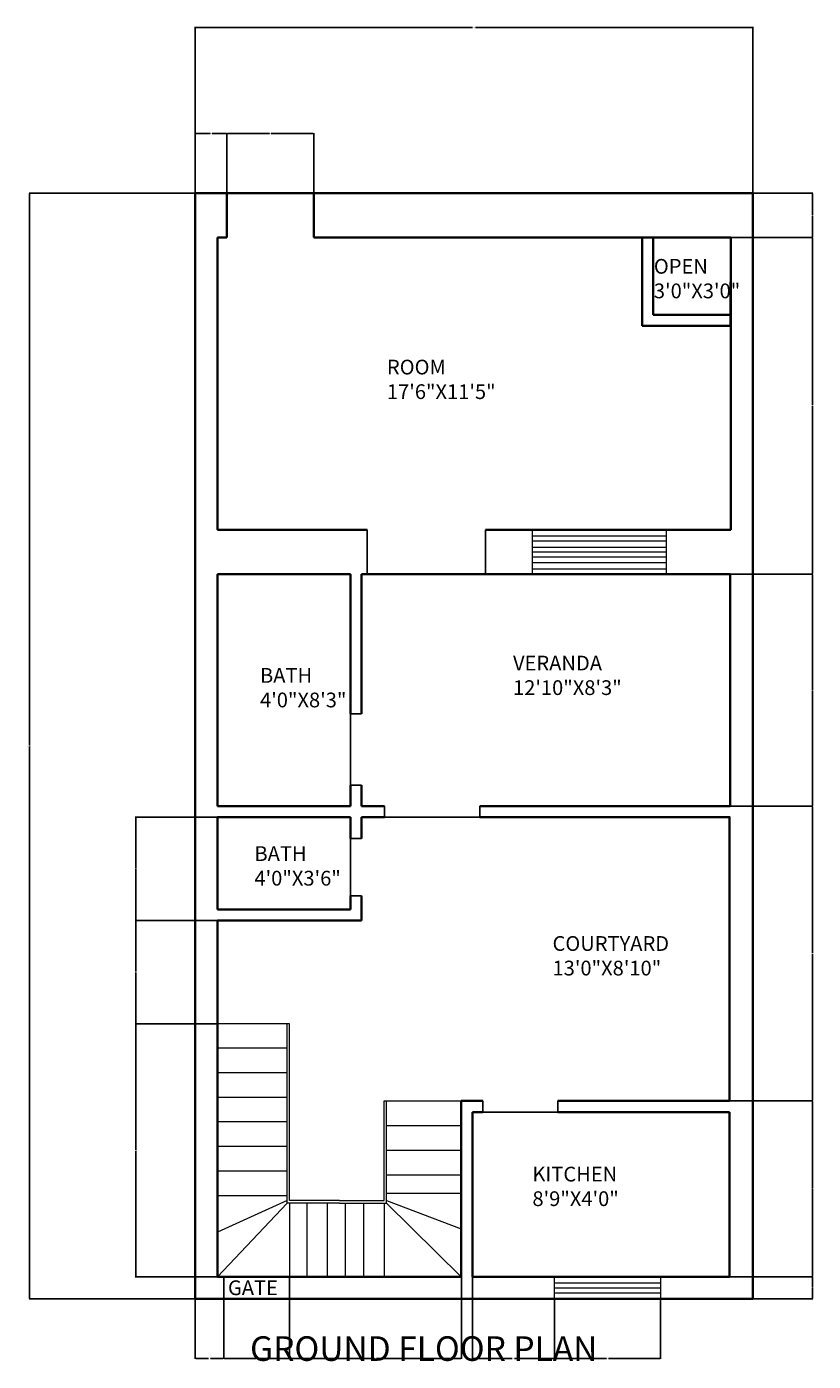
# Model space of a CAD drawing. Units: inches. Extents: x 2673 to 3344, y 1818 to 2362.
# Tile 1 of 2: x 2673 to 2994, y 1818 to 2362. Entities that reach past the tile are written whole.
import ezdxf

# ---------------------------------------------------------------- set-up
doc = ezdxf.new("R2010")
doc.units = ezdxf.units.IN
for name, color, linetype, lineweight in [('A-ANNO-DIMS', 2, 'Continuous', 18), ('A-ANNO-TEXT', 7, 'Continuous', 18), ('A-ANNO-TITL', 7, 'Continuous', 35), ('A-AREA-IDEN', 7, 'Continuous', 18), ('A-DOOR', 3, 'Continuous', 25), ('A-FLOR-STRS', 8, 'Continuous', 18), ('A-GLAZ', 4, 'Continuous', 18), ('A-WALL', 7, 'Continuous', 35)]:
    doc.layers.add(name, color=color, linetype=linetype, lineweight=lineweight)
doc.styles.get("Standard").update_dxf_attribs({"font": 'arial.ttf'})
doc.dimstyles.get("Standard").update_dxf_attribs({"dimtxt": 0.18, "dimasz": 0.18, "dimexe": 0.18, "dimexo": 0.0625, "dimgap": 0.09, "dimtad": 0, "dimtih": 1, "dimtoh": 1, "dimdec": 4, "dimzin": 0, "dimdsep": 46, "dimtxsty": 'Standard', "dimcen": 0.09, "dimadec": 0, "dimazin": 0, "dimtfac": 1, "dimtdec": 4, "dimtofl": 0, "dimtmove": 0, "dimatfit": 3, "dimfxl": 1, "dimtolj": 1, "dimtzin": 0, "dimarcsym": 0})

# ---------------------------------------------------------------- blocks, each defined once
blk = doc.blocks.new('FLOOR-PERIMETER-227X450')
for p, q in [((0, 450), (227, 450)), ((0, 0), (0, 450)), ((227, 450), (227, 0)), ((227, 0), (0, 0))]:
    blk.add_line(p, q)
blk = doc.blocks.new('*D2')
at = {"layer": 'A-ANNO-DIMS', "color": 0, "lineweight": -2, "transparency": 16777216}
for p, q in [((2742.07, 2293.79), (2674.46, 2293.79)), ((2674.64, 2293.61), (2674.64, 2068.98)), ((2674.64, 1843.97), (2674.64, 2068.61)), ((2742.07, 1843.79), (2674.46, 1843.79))]:
    blk.add_line(p, q, dxfattribs=at)
at = {"layer": 'A-ANNO-DIMS', "color": 0, "transparency": 16777216}
for points in [[(2674.61, 2293.61), (2674.67, 2293.61), (2674.64, 2293.79)], [(2674.61, 1843.97), (2674.67, 1843.97), (2674.64, 1843.79)]]:
    blk.add_solid(points, dxfattribs=at)
at = {"layer": 'Defpoints', "color": 0, "transparency": 16777216}
for p in [(2674.64, 2293.79), (2742.14, 2293.79), (2742.14, 1843.79)]:
    blk.add_point(p, dxfattribs=at)
at = {"layer": 'A-ANNO-DIMS', "color": 0, "transparency": 16777216, "insert": (2674.64, 2068.79), "char_height": 0.18, "attachment_point": 5}
blk.add_mtext('\\A1;FOOTPRINT 450 TYP.', dxfattribs=at)
blk = doc.blocks.new('*D3')
at = {"layer": 'A-ANNO-DIMS', "color": 0, "lineweight": -2, "transparency": 16777216}
for p, q in [((2742.14, 2293.86), (2742.14, 2361.47)), ((2742.32, 2361.29), (2855.04, 2361.29)), ((2968.96, 2361.29), (2856.24, 2361.29)), ((2969.14, 2293.86), (2969.14, 2361.47))]:
    blk.add_line(p, q, dxfattribs=at)
at = {"layer": 'A-ANNO-DIMS', "color": 0, "transparency": 16777216}
for points in [[(2742.32, 2361.32), (2742.32, 2361.26), (2742.14, 2361.29)], [(2968.96, 2361.32), (2968.96, 2361.26), (2969.14, 2361.29)]]:
    blk.add_solid(points, dxfattribs=at)
at = {"layer": 'Defpoints', "color": 0, "transparency": 16777216}
for p in [(2969.14, 2361.29), (2742.14, 2293.79), (2969.14, 2293.79)]:
    blk.add_point(p, dxfattribs=at)
at = {"layer": 'A-ANNO-DIMS', "color": 0, "transparency": 16777216, "insert": (2855.64, 2361.29), "char_height": 0.18, "attachment_point": 5}
blk.add_mtext('\\A1;227 TYP.', dxfattribs=at)
blk = doc.blocks.new('*D6')
at = {"layer": 'A-ANNO-DIMS', "color": 0, "lineweight": -2, "transparency": 16777216}
for p, q in [((2959.72, 1852.79), (2993.57, 1852.79)), ((2993.39, 1852.61), (2993.39, 1848.48)), ((2993.39, 1843.97), (2993.39, 1848.11)), ((2969.2, 1843.79), (2993.57, 1843.79))]:
    blk.add_line(p, q, dxfattribs=at)
at = {"layer": 'A-ANNO-DIMS', "color": 0, "transparency": 16777216}
for points in [[(2993.36, 1852.61), (2993.42, 1852.61), (2993.39, 1852.79)], [(2993.36, 1843.97), (2993.42, 1843.97), (2993.39, 1843.79)]]:
    blk.add_solid(points, dxfattribs=at)
at = {"layer": 'Defpoints', "color": 0, "transparency": 16777216}
for p in [(2959.65, 1852.79), (2993.39, 1852.79), (2969.14, 1843.79)]:
    blk.add_point(p, dxfattribs=at)
at = {"layer": 'A-ANNO-DIMS', "color": 0, "transparency": 16777216, "insert": (2993.39, 1848.29), "char_height": 0.18, "attachment_point": 5}
blk.add_mtext('\\A1;9', dxfattribs=at)
blk = doc.blocks.new('*D7')
at = {"layer": 'A-ANNO-DIMS', "color": 0, "lineweight": -2, "transparency": 16777216}
for p, q in [((2959.72, 1924.35), (2993.57, 1924.35)), ((2993.39, 1924.17), (2993.39, 1888.75)), ((2993.39, 1852.97), (2993.39, 1888.39)), ((2959.72, 1852.79), (2993.57, 1852.79))]:
    blk.add_line(p, q, dxfattribs=at)
at = {"layer": 'A-ANNO-DIMS', "color": 0, "transparency": 16777216}
for points in [[(2993.36, 1924.17), (2993.42, 1924.17), (2993.39, 1924.35)], [(2993.36, 1852.97), (2993.42, 1852.97), (2993.39, 1852.79)]]:
    blk.add_solid(points, dxfattribs=at)
at = {"layer": 'Defpoints', "color": 0, "transparency": 16777216}
for p in [(2959.65, 1924.35), (2993.39, 1924.35), (2959.65, 1852.79)]:
    blk.add_point(p, dxfattribs=at)
at = {"layer": 'A-ANNO-DIMS', "color": 0, "transparency": 16777216, "insert": (2993.39, 1888.57), "char_height": 0.18, "attachment_point": 5}
blk.add_mtext('\\A1;71.55', dxfattribs=at)
blk = doc.blocks.new('*D8')
at = {"layer": 'A-ANNO-DIMS', "color": 0, "lineweight": -2, "transparency": 16777216}
for p, q in [((2960.01, 2044.3), (2993.57, 2044.3)), ((2993.39, 2044.12), (2993.39, 1984.5)), ((2993.39, 1924.53), (2993.39, 1984.14)), ((2959.72, 1924.35), (2993.57, 1924.35))]:
    blk.add_line(p, q, dxfattribs=at)
at = {"layer": 'A-ANNO-DIMS', "color": 0, "transparency": 16777216}
for points in [[(2993.36, 2044.12), (2993.42, 2044.12), (2993.39, 2044.3)], [(2993.36, 1924.53), (2993.42, 1924.53), (2993.39, 1924.35)]]:
    blk.add_solid(points, dxfattribs=at)
at = {"layer": 'Defpoints', "color": 0, "transparency": 16777216}
for p in [(2959.95, 2044.3), (2993.39, 2044.3), (2959.65, 1924.35)]:
    blk.add_point(p, dxfattribs=at)
at = {"layer": 'A-ANNO-DIMS', "color": 0, "transparency": 16777216, "insert": (2993.39, 1984.32), "char_height": 0.18, "attachment_point": 5}
blk.add_mtext('\\A1;119.95', dxfattribs=at)
blk = doc.blocks.new('*D9')
at = {"layer": 'A-ANNO-DIMS', "color": 0, "lineweight": -2, "transparency": 16777216}
for p, q in [((2960.01, 2138.79), (2993.57, 2138.79)), ((2993.39, 2138.61), (2993.39, 2091.73)), ((2993.39, 2044.48), (2993.39, 2091.36)), ((2960.01, 2044.3), (2993.57, 2044.3))]:
    blk.add_line(p, q, dxfattribs=at)
at = {"layer": 'A-ANNO-DIMS', "color": 0, "transparency": 16777216}
for points in [[(2993.36, 2138.61), (2993.42, 2138.61), (2993.39, 2138.79)], [(2993.36, 2044.48), (2993.42, 2044.48), (2993.39, 2044.3)]]:
    blk.add_solid(points, dxfattribs=at)
at = {"layer": 'Defpoints', "color": 0, "transparency": 16777216}
for p in [(2959.95, 2138.79), (2993.39, 2138.79), (2959.95, 2044.3)]:
    blk.add_point(p, dxfattribs=at)
at = {"layer": 'A-ANNO-DIMS', "color": 0, "transparency": 16777216, "insert": (2993.39, 2091.55), "char_height": 0.18, "attachment_point": 5}
blk.add_mtext('\\A1;94.5', dxfattribs=at)
blk = doc.blocks.new('*D10')
at = {"layer": 'A-ANNO-DIMS', "color": 0, "lineweight": -2, "transparency": 16777216}
for p, q in [((2960.2, 2275.79), (2993.57, 2275.79)), ((2993.39, 2275.61), (2993.39, 2207.48)), ((2993.39, 2138.97), (2993.39, 2207.11)), ((2960.01, 2138.79), (2993.57, 2138.79))]:
    blk.add_line(p, q, dxfattribs=at)
at = {"layer": 'A-ANNO-DIMS', "color": 0, "transparency": 16777216}
for points in [[(2993.36, 2275.61), (2993.42, 2275.61), (2993.39, 2275.79)], [(2993.36, 2138.97), (2993.42, 2138.97), (2993.39, 2138.79)]]:
    blk.add_solid(points, dxfattribs=at)
at = {"layer": 'Defpoints', "color": 0, "transparency": 16777216}
for p in [(2960.14, 2275.79), (2993.39, 2275.79), (2959.95, 2138.79)]:
    blk.add_point(p, dxfattribs=at)
at = {"layer": 'A-ANNO-DIMS', "color": 0, "transparency": 16777216, "insert": (2993.39, 2207.29), "char_height": 0.18, "attachment_point": 5}
blk.add_mtext('\\A1;137', dxfattribs=at)
blk = doc.blocks.new('*D11')
at = {"layer": 'A-ANNO-DIMS', "color": 0, "lineweight": -2, "transparency": 16777216}
for p, q in [((2969.2, 2293.79), (2993.57, 2293.79)), ((2993.39, 2293.61), (2993.39, 2284.98)), ((2993.39, 2275.97), (2993.39, 2284.61)), ((2960.2, 2275.79), (2993.57, 2275.79))]:
    blk.add_line(p, q, dxfattribs=at)
at = {"layer": 'A-ANNO-DIMS', "color": 0, "transparency": 16777216}
for points in [[(2993.36, 2293.61), (2993.42, 2293.61), (2993.39, 2293.79)], [(2993.36, 2275.97), (2993.42, 2275.97), (2993.39, 2275.79)]]:
    blk.add_solid(points, dxfattribs=at)
at = {"layer": 'Defpoints', "color": 0, "transparency": 16777216}
for p in [(2969.14, 2293.79), (2993.39, 2293.79), (2960.14, 2275.79)]:
    blk.add_point(p, dxfattribs=at)
at = {"layer": 'A-ANNO-DIMS', "color": 0, "transparency": 16777216, "insert": (2993.39, 2284.79), "char_height": 0.18, "attachment_point": 5}
blk.add_mtext('\\A1;18', dxfattribs=at)
blk = doc.blocks.new('*D12')
at = {"layer": 'A-ANNO-DIMS', "color": 0, "lineweight": -2, "transparency": 16777216}
for p, q in [((2742.14, 1843.73), (2742.14, 1819.36)), ((2753.69, 1843.73), (2753.69, 1819.36)), ((2742.32, 1819.54), (2747.46, 1819.54)), ((2753.51, 1819.54), (2748.37, 1819.54))]:
    blk.add_line(p, q, dxfattribs=at)
at = {"layer": 'A-ANNO-DIMS', "color": 0, "transparency": 16777216}
for points in [[(2742.32, 1819.57), (2742.32, 1819.51), (2742.14, 1819.54)], [(2753.51, 1819.57), (2753.51, 1819.51), (2753.69, 1819.54)]]:
    blk.add_solid(points, dxfattribs=at)
at = {"layer": 'Defpoints', "color": 0, "transparency": 16777216}
for p in [(2742.14, 1843.79), (2753.69, 1843.79), (2753.69, 1819.54)]:
    blk.add_point(p, dxfattribs=at)
at = {"layer": 'A-ANNO-DIMS', "color": 0, "transparency": 16777216, "insert": (2747.91, 1819.54), "char_height": 0.18, "attachment_point": 5}
blk.add_mtext('\\A1;11.556', dxfattribs=at)
blk = doc.blocks.new('*D13')
at = {"layer": 'A-ANNO-DIMS', "color": 0, "lineweight": -2, "transparency": 16777216}
for p, q in [((2753.69, 1843.73), (2753.69, 1819.36)), ((2780.49, 1843.73), (2780.49, 1819.36)), ((2753.87, 1819.54), (2766.77, 1819.54)), ((2780.31, 1819.54), (2767.42, 1819.54))]:
    blk.add_line(p, q, dxfattribs=at)
at = {"layer": 'A-ANNO-DIMS', "color": 0, "transparency": 16777216}
for points in [[(2753.87, 1819.57), (2753.87, 1819.51), (2753.69, 1819.54)], [(2780.31, 1819.57), (2780.31, 1819.51), (2780.49, 1819.54)]]:
    blk.add_solid(points, dxfattribs=at)
at = {"layer": 'Defpoints', "color": 0, "transparency": 16777216}
for p in [(2753.69, 1843.79), (2780.49, 1843.79), (2780.49, 1819.54)]:
    blk.add_point(p, dxfattribs=at)
at = {"layer": 'A-ANNO-DIMS', "color": 0, "transparency": 16777216, "insert": (2767.09, 1819.54), "char_height": 0.18, "attachment_point": 5}
blk.add_mtext('\\A1;26.8', dxfattribs=at)
blk = doc.blocks.new('*D14')
at = {"layer": 'A-ANNO-DIMS', "color": 0, "lineweight": -2, "transparency": 16777216}
for p, q in [((2850.45, 1852.73), (2850.45, 1819.36)), ((2780.49, 1843.73), (2780.49, 1819.36)), ((2780.67, 1819.54), (2815.08, 1819.54)), ((2850.27, 1819.54), (2815.86, 1819.54))]:
    blk.add_line(p, q, dxfattribs=at)
at = {"layer": 'A-ANNO-DIMS', "color": 0, "transparency": 16777216}
for points in [[(2780.67, 1819.57), (2780.67, 1819.51), (2780.49, 1819.54)], [(2850.27, 1819.57), (2850.27, 1819.51), (2850.45, 1819.54)]]:
    blk.add_solid(points, dxfattribs=at)
at = {"layer": 'Defpoints', "color": 0, "transparency": 16777216}
for p in [(2850.45, 1852.79), (2780.49, 1843.79), (2850.45, 1819.54)]:
    blk.add_point(p, dxfattribs=at)
at = {"layer": 'A-ANNO-DIMS', "color": 0, "transparency": 16777216, "insert": (2815.47, 1819.54), "char_height": 0.18, "attachment_point": 5}
blk.add_mtext('\\A1;69.95', dxfattribs=at)
blk = doc.blocks.new('*D15')
at = {"layer": 'A-ANNO-DIMS', "color": 0, "lineweight": -2, "transparency": 16777216}
for p, q in [((2854.95, 1852.73), (2854.95, 1819.36)), ((2888.33, 1843.73), (2888.33, 1819.36)), ((2855.13, 1819.54), (2871.18, 1819.54)), ((2888.15, 1819.54), (2872.1, 1819.54))]:
    blk.add_line(p, q, dxfattribs=at)
at = {"layer": 'A-ANNO-DIMS', "color": 0, "transparency": 16777216}
for points in [[(2855.13, 1819.57), (2855.13, 1819.51), (2854.95, 1819.54)], [(2888.15, 1819.57), (2888.15, 1819.51), (2888.33, 1819.54)]]:
    blk.add_solid(points, dxfattribs=at)
at = {"layer": 'Defpoints', "color": 0, "transparency": 16777216}
for p in [(2854.95, 1852.79), (2888.33, 1843.79), (2888.33, 1819.54)]:
    blk.add_point(p, dxfattribs=at)
at = {"layer": 'A-ANNO-DIMS', "color": 0, "transparency": 16777216, "insert": (2871.64, 1819.54), "char_height": 0.18, "attachment_point": 5}
blk.add_mtext('\\A1;33.386', dxfattribs=at)
blk = doc.blocks.new('*D16')
at = {"layer": 'A-ANNO-DIMS', "color": 0, "lineweight": -2, "transparency": 16777216}
for p, q in [((2888.33, 1843.73), (2888.33, 1819.36)), ((2931.58, 1843.73), (2931.58, 1819.36)), ((2888.51, 1819.54), (2909.49, 1819.54)), ((2931.4, 1819.54), (2910.42, 1819.54))]:
    blk.add_line(p, q, dxfattribs=at)
at = {"layer": 'A-ANNO-DIMS', "color": 0, "transparency": 16777216}
for points in [[(2888.51, 1819.57), (2888.51, 1819.51), (2888.33, 1819.54)], [(2931.4, 1819.57), (2931.4, 1819.51), (2931.58, 1819.54)]]:
    blk.add_solid(points, dxfattribs=at)
at = {"layer": 'Defpoints', "color": 0, "transparency": 16777216}
for p in [(2888.33, 1843.79), (2931.58, 1843.79), (2931.58, 1819.54)]:
    blk.add_point(p, dxfattribs=at)
at = {"layer": 'A-ANNO-DIMS', "color": 0, "transparency": 16777216, "insert": (2909.96, 1819.54), "char_height": 0.18, "attachment_point": 5}
blk.add_mtext('\\A1;43.245', dxfattribs=at)
blk = doc.blocks.new('*D17')
at = {"layer": 'A-ANNO-DIMS', "color": 0, "lineweight": -2, "transparency": 16777216}
for p, q in [((2742.14, 2293.86), (2742.14, 2318.22)), ((2742.32, 2318.04), (2748.12, 2318.04)), ((2754.84, 2318.04), (2749.03, 2318.04)), ((2755.02, 2293.86), (2755.02, 2318.22))]:
    blk.add_line(p, q, dxfattribs=at)
at = {"layer": 'A-ANNO-DIMS', "color": 0, "transparency": 16777216}
for points in [[(2742.32, 2318.07), (2742.32, 2318.01), (2742.14, 2318.04)], [(2754.84, 2318.07), (2754.84, 2318.01), (2755.02, 2318.04)]]:
    blk.add_solid(points, dxfattribs=at)
at = {"layer": 'Defpoints', "color": 0, "transparency": 16777216}
for p in [(2755.02, 2318.04), (2742.14, 2293.79), (2755.02, 2293.79)]:
    blk.add_point(p, dxfattribs=at)
at = {"layer": 'A-ANNO-DIMS', "color": 0, "transparency": 16777216, "insert": (2748.58, 2318.04), "char_height": 0.18, "attachment_point": 5}
blk.add_mtext('\\A1;12.884', dxfattribs=at)
blk = doc.blocks.new('*D18')
at = {"layer": 'A-ANNO-DIMS', "color": 0, "lineweight": -2, "transparency": 16777216}
for p, q in [((2755.02, 2293.86), (2755.02, 2318.22)), ((2755.2, 2318.04), (2772.3, 2318.04)), ((2790.15, 2318.04), (2773.05, 2318.04)), ((2790.33, 2293.86), (2790.33, 2318.22))]:
    blk.add_line(p, q, dxfattribs=at)
at = {"layer": 'A-ANNO-DIMS', "color": 0, "transparency": 16777216}
for points in [[(2755.2, 2318.07), (2755.2, 2318.01), (2755.02, 2318.04)], [(2790.15, 2318.07), (2790.15, 2318.01), (2790.33, 2318.04)]]:
    blk.add_solid(points, dxfattribs=at)
at = {"layer": 'Defpoints', "color": 0, "transparency": 16777216}
for p in [(2790.33, 2318.04), (2755.02, 2293.79), (2790.33, 2293.79)]:
    blk.add_point(p, dxfattribs=at)
at = {"layer": 'A-ANNO-DIMS', "color": 0, "transparency": 16777216, "insert": (2772.68, 2318.04), "char_height": 0.18, "attachment_point": 5}
blk.add_mtext('\\A1;35.31', dxfattribs=at)
blk = doc.blocks.new('*D19')
at = {"layer": 'A-ANNO-DIMS', "color": 0, "lineweight": -2, "transparency": 16777216}
for p, q in [((2751.07, 1955.8), (2717.71, 1955.8)), ((2717.89, 1955.62), (2717.89, 1904.48)), ((2717.89, 1852.97), (2717.89, 1904.11)), ((2751.07, 1852.79), (2717.71, 1852.79))]:
    blk.add_line(p, q, dxfattribs=at)
at = {"layer": 'A-ANNO-DIMS', "color": 0, "transparency": 16777216}
for points in [[(2717.86, 1955.62), (2717.92, 1955.62), (2717.89, 1955.8)], [(2717.86, 1852.97), (2717.92, 1852.97), (2717.89, 1852.79)]]:
    blk.add_solid(points, dxfattribs=at)
at = {"layer": 'Defpoints', "color": 0, "transparency": 16777216}
for p in [(2717.89, 1955.8), (2751.14, 1955.8), (2751.14, 1852.79)]:
    blk.add_point(p, dxfattribs=at)
at = {"layer": 'A-ANNO-DIMS', "color": 0, "transparency": 16777216, "insert": (2717.89, 1904.3), "char_height": 0.18, "attachment_point": 5}
blk.add_mtext('\\A1;103', dxfattribs=at)
blk = doc.blocks.new('*D20')
at = {"layer": 'A-ANNO-DIMS', "color": 0, "lineweight": -2, "transparency": 16777216}
for p, q in [((2751.07, 1997.8), (2717.71, 1997.8)), ((2717.89, 1997.62), (2717.89, 1976.98)), ((2717.89, 1955.98), (2717.89, 1976.62)), ((2751.07, 1955.8), (2717.71, 1955.8))]:
    blk.add_line(p, q, dxfattribs=at)
at = {"layer": 'A-ANNO-DIMS', "color": 0, "transparency": 16777216}
for points in [[(2717.86, 1997.62), (2717.92, 1997.62), (2717.89, 1997.8)], [(2717.86, 1955.98), (2717.92, 1955.98), (2717.89, 1955.8)]]:
    blk.add_solid(points, dxfattribs=at)
at = {"layer": 'Defpoints', "color": 0, "transparency": 16777216}
for p in [(2717.89, 1997.8), (2751.14, 1997.8), (2751.14, 1955.8)]:
    blk.add_point(p, dxfattribs=at)
at = {"layer": 'A-ANNO-DIMS', "color": 0, "transparency": 16777216, "insert": (2717.89, 1976.8), "char_height": 0.18, "attachment_point": 5}
blk.add_mtext('\\A1;42', dxfattribs=at)
blk = doc.blocks.new('*D21')
at = {"layer": 'A-ANNO-DIMS', "color": 0, "lineweight": -2, "transparency": 16777216}
for p, q in [((2751.07, 2039.8), (2717.71, 2039.8)), ((2717.89, 2039.62), (2717.89, 2018.98)), ((2717.89, 1997.98), (2717.89, 2018.62)), ((2751.07, 1997.8), (2717.71, 1997.8))]:
    blk.add_line(p, q, dxfattribs=at)
at = {"layer": 'A-ANNO-DIMS', "color": 0, "transparency": 16777216}
for points in [[(2717.86, 2039.62), (2717.92, 2039.62), (2717.89, 2039.8)], [(2717.86, 1997.98), (2717.92, 1997.98), (2717.89, 1997.8)]]:
    blk.add_solid(points, dxfattribs=at)
at = {"layer": 'Defpoints', "color": 0, "transparency": 16777216}
for p in [(2717.89, 2039.8), (2751.14, 2039.8), (2751.14, 1997.8)]:
    blk.add_point(p, dxfattribs=at)
at = {"layer": 'A-ANNO-DIMS', "color": 0, "transparency": 16777216, "insert": (2717.89, 2018.8), "char_height": 0.18, "attachment_point": 5}
blk.add_mtext('\\A1;42', dxfattribs=at)

msp = doc.modelspace()

# ---------------------------------------------------------------- linework, layer by layer
at = {"layer": 'A-DOOR'}
for p, q in [((2812.0877, 2138.7941), (2812.0877, 2156.7941)), ((2860.2455, 2138.7941), (2860.2455, 2156.7941)), ((2805.3617, 2081.8721), (2809.8617, 2081.8721)), ((2805.3617, 2081.8721), (2805.3617, 2052.8408)), ((2805.3617, 2052.8408), (2809.8617, 2052.8408)), ((2819.1101, 2039.7972), (2819.1101, 2044.2972)), ((2857.9709, 2039.7972), (2857.9709, 2044.2972)), ((2819.1101, 2039.7972), (2857.9709, 2039.7972)), ((2805.3617, 2031.1818), (2809.8617, 2031.1818)), ((2805.3617, 2007.8792), (2805.3617, 2031.1818)), ((2805.3617, 2007.8792), (2809.8617, 2007.8792)), ((2859.1524, 1919.8472), (2859.1524, 1924.3472)), ((2889.7363, 1919.8472), (2889.7363, 1924.3472)), ((2859.1524, 1919.8472), (2890.9676, 1919.8472)), ((2753.6928, 1852.7936), (2753.6928, 1843.7936)), ((2780.4931, 1852.7936), (2780.4931, 1843.7936))]:
    msp.add_line(p, q, dxfattribs=at)
at = {"layer": 'A-FLOR-STRS'}
for p, q in [((2780.4931, 1955.7975), (2751.137, 1955.7975)), ((2779.4931, 1924.3472), (2779.4931, 1955.7975)), ((2780.4931, 1924.3472), (2780.4931, 1955.7975)), ((2779.4931, 1945.7975), (2751.137, 1945.7975)), ((2779.4931, 1935.7975), (2751.137, 1935.7975)), ((2779.4931, 1925.7975), (2751.137, 1925.7975)), ((2779.4931, 1882.7728), (2779.4931, 1924.3472)), ((2780.4931, 1883.7728), (2780.4931, 1924.3472)), ((2818.9849, 1883.7728), (2818.9849, 1924.3472)), ((2818.9849, 1924.3472), (2819.9849, 1924.3472)), ((2819.9849, 1882.7728), (2819.9849, 1924.3472)), ((2819.9849, 1924.3472), (2850.4469, 1924.3472)), ((2779.4931, 1915.7975), (2751.137, 1915.7975)), ((2819.9849, 1914.3472), (2850.4469, 1914.3472)), ((2779.4931, 1905.7975), (2751.137, 1905.7975)), ((2819.9849, 1904.3472), (2850.4469, 1904.3472)), ((2779.4931, 1895.7975), (2751.137, 1895.7975)), ((2819.9849, 1894.3472), (2850.4469, 1894.3472)), ((2779.4931, 1885.7975), (2751.137, 1885.7975)), ((2819.9849, 1886.8433), (2850.4469, 1886.8433)), ((2779.4931, 1883.7728), (2751.137, 1870.992)), ((2779.4931, 1882.7728), (2751.137, 1852.7936)), ((2800.792, 1882.7728), (2779.4931, 1882.7728)), ((2800.792, 1883.7728), (2780.4931, 1883.7728)), ((2780.4931, 1882.7728), (2780.4931, 1852.7936)), ((2787.7372, 1852.7936), (2787.7372, 1882.7728)), ((2795.9322, 1852.7936), (2795.9322, 1882.7728)), ((2800.792, 1883.7728), (2818.9849, 1883.7728)), ((2800.792, 1882.7728), (2819.9849, 1882.7728)), ((2803.2385, 1852.7936), (2803.2385, 1882.7728)), ((2810.7424, 1852.7936), (2810.7424, 1882.7728)), ((2818.9849, 1882.7728), (2818.9849, 1852.7936)), ((2819.9849, 1883.7728), (2850.4469, 1872.2734)), ((2819.9849, 1882.7728), (2850.4469, 1852.7907))]:
    msp.add_line(p, q, dxfattribs=at)
at = {"layer": 'A-GLAZ'}
for p, q in [((2879.3937, 2154.389), (2933.8124, 2154.389)), ((2879.3937, 2152.3252), (2933.8124, 2152.3252)), ((2879.3937, 2149.7455), (2933.8124, 2149.7455)), ((2879.3937, 2147.7941), (2933.8124, 2147.7941)), ((2879.3937, 2145.8621), (2933.8124, 2145.8621)), ((2879.3937, 2143.5352), (2933.8124, 2143.5352)), ((2879.3937, 2140.8851), (2933.8124, 2140.8851)), ((2888.3325, 1850.2838), (2931.5776, 1850.3475)), ((2888.3325, 1848.2936), (2931.5776, 1848.2936)), ((2888.3325, 1846.2746), (2931.5776, 1846.2746))]:
    msp.add_line(p, q, dxfattribs=at)
for points in [[(2879.3937, 2156.7941), (2933.8124, 2156.7941), (2933.8124, 2138.7941), (2879.3937, 2138.7941)], [(2888.3325, 1852.7936), (2931.5776, 1852.7936), (2931.5776, 1843.7936), (2888.3325, 1843.7936)]]:
    msp.add_lwpolyline(points, close=True, dxfattribs=at)
at = {"layer": 'A-WALL'}
for p, q in [((2755.0211, 2275.7936), (2755.0211, 2293.7936)), ((2790.3344, 2275.7936), (2790.3344, 2293.7936)), ((2751.137, 2275.7936), (2755.0211, 2275.7936)), ((2751.137, 2156.7941), (2751.137, 2275.7936)), ((2790.3344, 2275.7936), (2960.137, 2275.7936)), ((2924.0554, 2239.7937), (2924.0554, 2275.7936)), ((2928.5554, 2244.2937), (2928.5554, 2275.7936)), ((2960.137, 2275.7936), (2960.0554, 2239.7937)), ((2960.137, 2275.7936), (2960.137, 2156.7941)), ((2960.0554, 2244.2937), (2928.5554, 2244.2937)), ((2960.0554, 2239.7937), (2924.0554, 2239.7937)), ((2809.4189, 2156.7941), (2751.137, 2156.7941)), ((2809.8617, 2156.7941), (2809.4189, 2156.7941)), ((2812.0877, 2156.7941), (2809.8617, 2156.7941)), ((2959.7568, 2156.7941), (2860.2455, 2156.7941)), ((2959.7568, 2156.7941), (2960.137, 2156.7941)), ((2805.3617, 2138.7941), (2751.137, 2138.7941)), ((2751.137, 2044.2972), (2751.137, 2138.7941)), ((2805.3617, 2081.8721), (2805.3617, 2138.7941)), ((2809.8617, 2138.7941), (2860.2455, 2138.7941)), ((2809.8617, 2081.8721), (2809.8617, 2138.7941)), ((2959.7568, 2138.7941), (2860.2455, 2138.7941)), ((2959.7568, 2138.7941), (2959.9469, 2138.7941)), ((2959.9469, 2138.7941), (2959.9469, 2044.2972)), ((2805.3617, 2044.2972), (2805.3617, 2052.8408)), ((2809.8617, 2044.2972), (2809.8617, 2052.8408)), ((2805.3617, 2044.2972), (2751.137, 2044.2972)), ((2819.1101, 2044.2972), (2809.8617, 2044.2972)), ((2959.3617, 2044.2972), (2857.9709, 2044.2972)), ((2959.3617, 2044.2972), (2959.9469, 2044.2972)), ((2805.3617, 2039.7972), (2751.137, 2039.7972)), ((2751.137, 2002.2983), (2751.137, 2039.7972)), ((2805.3617, 2039.7972), (2805.3617, 2031.1818)), ((2809.8617, 2039.7972), (2809.8617, 2031.1818)), ((2819.1101, 2039.7972), (2809.8617, 2039.7972)), ((2959.3617, 2039.7972), (2857.9709, 2039.7972)), ((2959.3617, 2039.7972), (2959.9469, 2039.7972)), ((2959.6543, 2039.7972), (2959.6543, 1924.3472)), ((2805.3617, 2007.8792), (2805.3617, 2002.2983)), ((2809.8617, 2007.8792), (2809.8617, 1997.7983)), ((2805.0541, 2002.2983), (2751.137, 2002.2983)), ((2805.0541, 2002.2983), (2805.3617, 2002.2983)), ((2751.137, 1852.7936), (2751.137, 1997.7983)), ((2805.0541, 1997.7983), (2751.137, 1997.7983)), ((2805.0541, 1997.7983), (2805.3617, 1997.7983)), ((2805.3617, 1997.7983), (2809.8617, 1997.7983)), ((2850.4469, 1919.8472), (2850.4469, 1924.3472)), ((2859.1524, 1924.3472), (2850.4469, 1924.3472)), ((2959.6543, 1924.3472), (2889.7363, 1924.3472)), ((2850.4469, 1852.7907), (2850.4469, 1919.8472)), ((2854.9469, 1852.7907), (2854.9469, 1919.8472)), ((2859.1524, 1919.8472), (2854.9469, 1919.8472)), ((2959.6543, 1919.8472), (2889.7363, 1919.8472)), ((2959.6543, 1919.8472), (2959.6543, 1852.7936)), ((2850.4469, 1852.7936), (2751.137, 1852.7936)), ((2959.6543, 1852.7936), (2854.9469, 1852.7936))]:
    msp.add_line(p, q, dxfattribs=at)

# ---------------------------------------------------------------- block references
msp.add_blockref('FLOOR-PERIMETER-227X450', (2742.137, 1843.7936), dxfattribs=at)

# ---------------------------------------------------------------- texts
at = {"layer": 'A-ANNO-TEXT', "insert": (2755.4278, 1851.3267), "char_height": 6, "attachment_point": 1}
msp.add_mtext_dynamic_manual_height_columns('GATE\\P ', width=4.95123, gutter_width=12.5, heights=[0], dxfattribs=at)
at = {"layer": 'A-ANNO-TITL', "insert": (2764.4221, 1828.5696), "char_height": 10, "attachment_point": 1}
msp.add_mtext_dynamic_manual_height_columns('GROUND FLOOR PLAN ', width=156.994222, gutter_width=12.5, heights=[0], dxfattribs=at)
at = {"layer": 'A-AREA-IDEN', "char_height": 6, "attachment_point": 1}
for s, width, insert in [('OPEN\\P3\'0"X3\'0"', 7.792091, (2928.8408, 2267.0357)), ('ROOM \\P17\'6"X11\'5"', 44.612926, (2820.1518, 2226.0263)), ('VERANDA\\P12\'10"X8\'3"', 37.705968, (2871.4973, 2105.5668)), ('BATH\\P4\'0"X8\'3"', 10.849641, (2768.4898, 2100.5464)), ('BATH\\P4\'0"X3\'6"', 10.849641, (2766.2121, 2028.0119)), ('COURTYARD\\P13\'0"X8\'10"', 22.904962, (2887.5788, 1991.4332)), ('KITCHEN \\P8\'9"X4\'0"', 28.845327, (2879.3946, 1897.579))]:
    msp.add_mtext_dynamic_manual_height_columns(s, width=width, gutter_width=12.5, heights=[0], dxfattribs=dict(at, insert=insert))

# ---------------------------------------------------------------- dimensions: what is measured, and where the dimension line sits
at = {"layer": 'A-ANNO-DIMS'}
dim = msp.add_linear_dim(base=(2969.137, 2361.2936), p1=(2742.137, 2293.7936), p2=(2969.137, 2293.7936), text='<> TYP.', dimstyle='Standard', override={"dimdec": 0, "dimlfac": 1, "dimrnd": 0, "dimzin": 0, "dimdsep": 46, "dimlunit": 2}, dxfattribs=at)
dim.commit()
dim.dimension.update_dxf_attribs({"geometry": '*D3', "text_midpoint": (2855.637, 2361.2936)})
for base, p1, p2, override, picture, middle in [((2755.0211, 2318.0436), (2742.137, 2293.7936), (2755.0211, 2293.7936), {"dimdec": 3, "dimlfac": 1, "dimrnd": 0, "dimzin": 0, "dimdsep": 46, "dimlunit": 2}, '*D17', (2748.5791, 2318.0436)), ((2790.3344, 2318.0436), (2755.0211, 2293.7936), (2790.3344, 2293.7936), {"dimdec": 2, "dimlfac": 1, "dimrnd": 0, "dimzin": 0, "dimdsep": 46, "dimlunit": 2}, '*D18', (2772.6777, 2318.0436)), ((2850.4469, 1819.5436), (2780.4931, 1843.7936), (2850.4469, 1852.7907), {"dimdec": 2, "dimlfac": 1, "dimrnd": 0, "dimzin": 0, "dimdsep": 46, "dimlunit": 2}, '*D14', (2815.47, 1819.5436)), ((2888.3325, 1819.5436), (2854.9469, 1852.7907), (2888.3325, 1843.7936), {"dimdec": 3, "dimlfac": 1, "dimrnd": 0, "dimzin": 0, "dimdsep": 46, "dimlunit": 2}, '*D15', (2871.6397, 1819.5436)), ((2753.6928, 1819.5436), (2742.137, 1843.7936), (2753.6928, 1843.7936), {"dimdec": 3, "dimlfac": 1, "dimrnd": 0, "dimzin": 0, "dimdsep": 46, "dimlunit": 2}, '*D12', (2747.9149, 1819.5436)), ((2780.4931, 1819.5436), (2753.6928, 1843.7936), (2780.4931, 1843.7936), {"dimdec": 1, "dimlfac": 1, "dimrnd": 0, "dimzin": 0, "dimdsep": 46, "dimlunit": 2}, '*D13', (2767.0929, 1819.5436)), ((2931.5776, 1819.5436), (2888.3325, 1843.7936), (2931.5776, 1843.7936), {"dimdec": 3, "dimlfac": 1, "dimrnd": 0, "dimzin": 0, "dimdsep": 46, "dimlunit": 2}, '*D16', (2909.955, 1819.5436))]:
    dim = msp.add_linear_dim(base=base, p1=p1, p2=p2, dimstyle='Standard', override=override, dxfattribs=at)
    dim.commit()
    dim.dimension.update_dxf_attribs({"geometry": picture, "text_midpoint": middle})
dim = msp.add_linear_dim(base=(2674.637, 2293.7936), p1=(2742.137, 1843.7936), p2=(2742.137, 2293.7936), angle=90, text='FOOTPRINT <> TYP.', dimstyle='Standard', override={"dimdec": 0, "dimlfac": 1, "dimrnd": 0, "dimzin": 0, "dimdsep": 46, "dimlunit": 2}, dxfattribs=at)
dim.commit()
dim.dimension.update_dxf_attribs({"geometry": '*D2', "text_midpoint": (2674.637, 2068.7936)})
for base, p1, p2, override, picture, middle in [((2993.387, 2293.7936), (2960.137, 2275.7936), (2969.137, 2293.7936), {"dimdec": 0, "dimlfac": 1, "dimrnd": 0, "dimzin": 0, "dimdsep": 46, "dimlunit": 2}, '*D11', (2993.387, 2284.7936)), ((2993.387, 2275.7936), (2959.9469, 2138.7941), (2960.137, 2275.7936), {"dimdec": 0, "dimlfac": 1, "dimrnd": 0, "dimzin": 0, "dimdsep": 46, "dimlunit": 2}, '*D10', (2993.387, 2207.2939)), ((2993.387, 2138.7941), (2959.9469, 2044.2972), (2959.9469, 2138.7941), {"dimdec": 1, "dimlfac": 1, "dimrnd": 0, "dimzin": 0, "dimdsep": 46, "dimlunit": 2}, '*D9', (2993.387, 2091.5457)), ((2993.387, 2044.2972), (2959.6543, 1924.3472), (2959.9469, 2044.2972), {"dimdec": 2, "dimlfac": 1, "dimrnd": 0, "dimzin": 0, "dimdsep": 46, "dimlunit": 2}, '*D8', (2993.387, 1984.3222)), ((2717.887, 2039.7972), (2751.137, 1997.7983), (2751.137, 2039.7972), {"dimdec": 0, "dimlfac": 1, "dimrnd": 0, "dimzin": 0, "dimdsep": 46, "dimlunit": 2}, '*D21', (2717.887, 2018.7977)), ((2717.887, 1997.7983), (2751.137, 1955.7975), (2751.137, 1997.7983), {"dimdec": 0, "dimlfac": 1, "dimrnd": 0, "dimzin": 0, "dimdsep": 46, "dimlunit": 2}, '*D20', (2717.887, 1976.7979)), ((2717.887, 1955.7975), (2751.137, 1852.7936), (2751.137, 1955.7975), {"dimdec": 0, "dimlfac": 1, "dimrnd": 0, "dimzin": 0, "dimdsep": 46, "dimlunit": 2}, '*D19', (2717.887, 1904.2956)), ((2993.387, 1924.3472), (2959.6543, 1852.7936), (2959.6543, 1924.3472), {"dimdec": 2, "dimlfac": 1, "dimrnd": 0, "dimzin": 0, "dimdsep": 46, "dimlunit": 2}, '*D7', (2993.387, 1888.5704)), ((2993.387, 1852.7936), (2969.137, 1843.7936), (2959.6543, 1852.7936), {"dimdec": 0, "dimlfac": 1, "dimrnd": 0, "dimzin": 0, "dimdsep": 46, "dimlunit": 2}, '*D6', (2993.387, 1848.2936))]:
    dim = msp.add_linear_dim(base=base, p1=p1, p2=p2, angle=90, dimstyle='Standard', override=override, dxfattribs=at)
    dim.commit()
    dim.dimension.update_dxf_attribs({"geometry": picture, "text_midpoint": middle})

doc.saveas('drawing.dxf')
